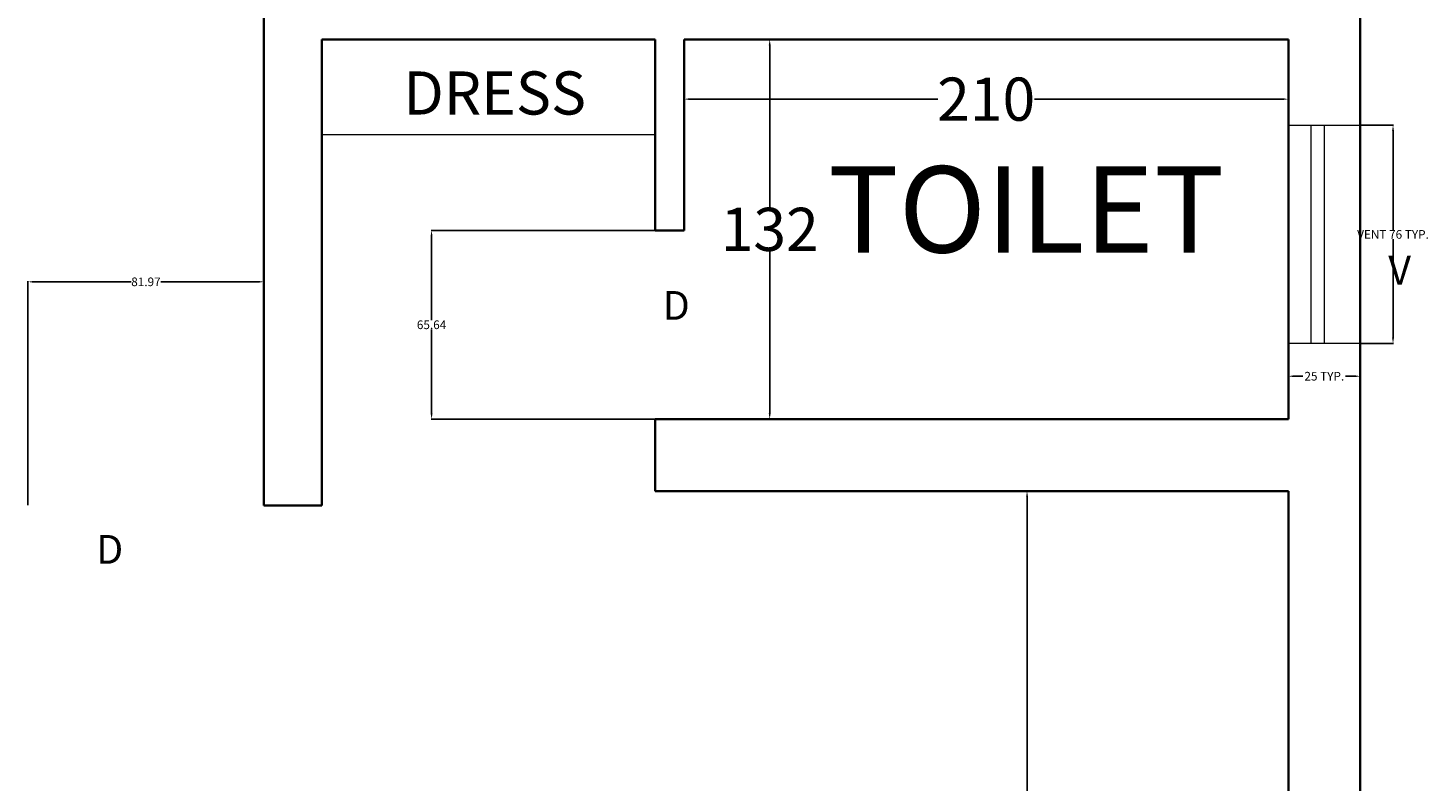
# Model space of a CAD drawing. Units: centimetres. Extents: x -121 to 3851, y -16 to 1180.
# Tile 15 of 16: x 3304 to 3791, y 320 to 582. Entities that reach past the tile are written whole.
import ezdxf

# ---------------------------------------------------------------- set-up
doc = ezdxf.new("R2010")
doc.units = ezdxf.units.CM
doc.header["$MEASUREMENT"] = 0
for name, color, linetype, lineweight in [('A-ANNO-DIMS', 2, 'Continuous', 18), ('A-ANNO-IDEN', 3, 'Continuous', 13), ('A-AREA-IDEN', 3, 'Continuous', 18), ('A-FLOR-CASE', 9, 'Continuous', 18), ('A-GLAZ', 4, 'Continuous', 18), ('A-WALL', 7, 'Continuous', 35)]:
    doc.layers.add(name, color=color, linetype=linetype, lineweight=lineweight)
doc.styles.get("Standard").update_dxf_attribs({"font": 'arial.ttf'})
doc.dimstyles.get("Standard").update_dxf_attribs({"dimtxt": 3, "dimasz": 2, "dimexe": 0.18, "dimexo": 0.0625, "dimgap": 0.09, "dimtad": 0, "dimtih": 1, "dimtoh": 1, "dimdec": 0, "dimzin": 0, "dimdsep": 46, "dimtxsty": 'Standard', "dimcen": 0.09, "dimadec": 0, "dimazin": 0, "dimtfac": 1, "dimtdec": 0, "dimtofl": 0, "dimtmove": 0, "dimatfit": 3, "dimfxl": 1, "dimtolj": 1, "dimtzin": 0, "dimarcsym": 0})

# ---------------------------------------------------------------- blocks, each defined once
blk = doc.blocks.new('*D14')
at = {"layer": 'A-ANNO-DIMS', "color": 0, "lineweight": -2, "transparency": 16777216}
for p, q in [((3562.02, 575.72), (3562.02, 519.48)), ((3562.09, 577.72), (3562.2, 577.72)), ((3562.02, 447.72), (3562.02, 503.97)), ((3562.09, 445.72), (3562.2, 445.72))]:
    blk.add_line(p, q, dxfattribs=at)
at = {"layer": 'A-ANNO-DIMS', "color": 0, "transparency": 16777216}
for points in [[(3561.69, 575.72), (3562.36, 575.72), (3562.02, 577.72)], [(3561.69, 447.72), (3562.36, 447.72), (3562.02, 445.72)]]:
    blk.add_solid(points, dxfattribs=at)
at = {"layer": 'Defpoints', "color": 0, "transparency": 16777216}
for p in [(3562.02, 577.72), (3562.02, 445.72), (3562.02, 445.72)]:
    blk.add_point(p, dxfattribs=at)
at = {"layer": 'A-ANNO-DIMS', "color": 0, "transparency": 16777216, "insert": (3562.02, 511.72), "char_height": 3, "attachment_point": 5}
blk.add_mtext('\\A1;{\\H5x;132}', dxfattribs=at)
blk = doc.blocks.new('*D15')
at = {"layer": 'A-ANNO-DIMS', "color": 0, "lineweight": -2, "transparency": 16777216}
for p, q in [((3532.26, 552.16), (3532.26, 557.17)), ((3534.26, 556.99), (3620.5, 556.99)), ((3740.26, 556.99), (3654.03, 556.99)), ((3742.26, 552.16), (3742.26, 557.17))]:
    blk.add_line(p, q, dxfattribs=at)
at = {"layer": 'A-ANNO-DIMS', "color": 0, "transparency": 16777216}
for points in [[(3534.26, 557.33), (3534.26, 556.66), (3532.26, 556.99)], [(3740.26, 557.33), (3740.26, 556.66), (3742.26, 556.99)]]:
    blk.add_solid(points, dxfattribs=at)
at = {"layer": 'Defpoints', "color": 0, "transparency": 16777216}
for p in [(3742.26, 556.99), (3532.26, 552.1), (3742.26, 552.1)]:
    blk.add_point(p, dxfattribs=at)
at = {"layer": 'A-ANNO-DIMS', "color": 0, "transparency": 16777216, "insert": (3637.26, 556.99), "char_height": 3, "attachment_point": 5}
blk.add_mtext('\\A1;{\\H5x;210}', dxfattribs=at)
blk = doc.blocks.new('*D17')
at = {"layer": 'A-ANNO-DIMS', "color": 0, "lineweight": -2, "transparency": 16777216}
for p, q in [((3651.46, 418.72), (3651.46, 281.03)), ((3651.53, 420.72), (3651.64, 420.72)), ((3651.46, 122.72), (3651.46, 260.41)), ((3651.53, 120.72), (3651.64, 120.72))]:
    blk.add_line(p, q, dxfattribs=at)
at = {"layer": 'A-ANNO-DIMS', "color": 0, "transparency": 16777216}
for points in [[(3651.13, 418.72), (3651.8, 418.72), (3651.46, 420.72)], [(3651.13, 122.72), (3651.8, 122.72), (3651.46, 120.72)]]:
    blk.add_solid(points, dxfattribs=at)
at = {"layer": 'Defpoints', "color": 0, "transparency": 16777216}
for p in [(3651.46, 420.72), (3651.46, 120.72), (3651.46, 120.72)]:
    blk.add_point(p, dxfattribs=at)
at = {"layer": 'A-ANNO-DIMS', "color": 0, "transparency": 16777216, "insert": (3651.46, 270.72), "char_height": 3, "attachment_point": 5}
blk.add_mtext('\\A1;{\\H6.66667x;300}', dxfattribs=at)
blk = doc.blocks.new('VENT-76CM')
for p, q in [((7.77, 75.86), (7.77, 0)), ((12.5, 75.86), (12.5, 0))]:
    blk.add_line(p, q)
blk.add_lwpolyline([(0, 75.86), (25, 75.86), (25, 0), (0, 0)], close=True)
blk = doc.blocks.new('*D31')
at = {"layer": 'A-ANNO-DIMS', "color": 0, "lineweight": -2, "transparency": 16777216}
for p, q in [((3767.33, 547.9), (3778.82, 547.9)), ((3778.64, 545.9), (3778.64, 511.59)), ((3778.64, 474.03), (3778.64, 508.34)), ((3767.33, 472.03), (3778.82, 472.03))]:
    blk.add_line(p, q, dxfattribs=at)
at = {"layer": 'A-ANNO-DIMS', "color": 0, "transparency": 16777216}
for points in [[(3778.31, 545.9), (3778.98, 545.9), (3778.64, 547.9)], [(3778.31, 474.03), (3778.98, 474.03), (3778.64, 472.03)]]:
    blk.add_solid(points, dxfattribs=at)
at = {"layer": 'Defpoints', "color": 0, "transparency": 16777216}
for p in [(3767.26, 547.9), (3778.64, 547.9), (3767.26, 472.03)]:
    blk.add_point(p, dxfattribs=at)
at = {"layer": 'A-ANNO-DIMS', "color": 0, "transparency": 16777216, "insert": (3778.64, 509.96), "char_height": 3, "attachment_point": 5}
blk.add_mtext('\\A1;VENT 76 TYP.', dxfattribs=at)
blk = doc.blocks.new('*D32')
at = {"layer": 'A-ANNO-DIMS', "color": 0, "lineweight": -2, "transparency": 16777216}
for p, q in [((3742.26, 471.97), (3742.26, 460.47)), ((3767.26, 471.97), (3767.26, 460.47)), ((3744.26, 460.65), (3747.35, 460.65)), ((3765.26, 460.65), (3762.18, 460.65))]:
    blk.add_line(p, q, dxfattribs=at)
at = {"layer": 'A-ANNO-DIMS', "color": 0, "transparency": 16777216}
for points in [[(3744.26, 460.99), (3744.26, 460.32), (3742.26, 460.65)], [(3765.26, 460.99), (3765.26, 460.32), (3767.26, 460.65)]]:
    blk.add_solid(points, dxfattribs=at)
at = {"layer": 'Defpoints', "color": 0, "transparency": 16777216}
for p in [(3742.26, 472.03), (3767.26, 472.03), (3767.26, 460.65)]:
    blk.add_point(p, dxfattribs=at)
at = {"layer": 'A-ANNO-DIMS', "color": 0, "transparency": 16777216, "insert": (3754.76, 460.65), "char_height": 3, "attachment_point": 5}
blk.add_mtext('\\A1;25 TYP.', dxfattribs=at)
blk = doc.blocks.new('*D72')
at = {"layer": 'A-ANNO-DIMS', "color": 0, "lineweight": -2, "transparency": 16777216}
for p, q in [((3304.26, 415.79), (3304.26, 493.65)), ((3306.26, 493.47), (3340.1, 493.47)), ((3384.23, 493.47), (3350.4, 493.47)), ((3386.23, 415.79), (3386.23, 493.65))]:
    blk.add_line(p, q, dxfattribs=at)
at = {"layer": 'A-ANNO-DIMS', "color": 0, "transparency": 16777216}
for points in [[(3306.26, 493.81), (3306.26, 493.14), (3304.26, 493.47)], [(3384.23, 493.81), (3384.23, 493.14), (3386.23, 493.47)]]:
    blk.add_solid(points, dxfattribs=at)
at = {"layer": 'Defpoints', "color": 0, "transparency": 16777216}
for p in [(3386.23, 493.47), (3304.26, 415.72), (3386.23, 415.72)]:
    blk.add_point(p, dxfattribs=at)
at = {"layer": 'A-ANNO-DIMS', "color": 0, "transparency": 16777216, "insert": (3345.25, 493.47), "char_height": 3, "attachment_point": 5}
blk.add_mtext('\\A1;81.97', dxfattribs=at)
blk = doc.blocks.new('*D80')
at = {"layer": 'A-ANNO-DIMS', "color": 0, "lineweight": -2, "transparency": 16777216}
for p, q in [((3522.2, 511.36), (3444.33, 511.36)), ((3444.51, 509.36), (3444.51, 480.17)), ((3444.51, 447.72), (3444.51, 476.92)), ((3522.2, 445.72), (3444.33, 445.72))]:
    blk.add_line(p, q, dxfattribs=at)
at = {"layer": 'A-ANNO-DIMS', "color": 0, "transparency": 16777216}
for points in [[(3444.18, 509.36), (3444.85, 509.36), (3444.51, 511.36)], [(3444.18, 447.72), (3444.85, 447.72), (3444.51, 445.72)]]:
    blk.add_solid(points, dxfattribs=at)
at = {"layer": 'Defpoints', "color": 0, "transparency": 16777216}
for p in [(3444.51, 511.36), (3522.26, 511.36), (3522.26, 445.72)]:
    blk.add_point(p, dxfattribs=at)
at = {"layer": 'A-ANNO-DIMS', "color": 0, "transparency": 16777216, "insert": (3444.51, 478.54), "char_height": 3, "attachment_point": 5}
blk.add_mtext('\\A1;65.64', dxfattribs=at)

msp = doc.modelspace()

# ---------------------------------------------------------------- linework, layer by layer
at = {"layer": 'A-FLOR-CASE'}
msp.add_line((3522.2642, 544.5435), (3406.327, 544.5435), dxfattribs=at)
at = {"layer": 'A-WALL'}
for p, q in [((3767.2642, 911.7228), (3767.2642, 95.7228)), ((3406.327, 577.7228), (3522.2642, 577.7228)), ((3522.2642, 577.7228), (3522.2642, 511.3642)), ((3532.2642, 577.7228), (3742.2642, 577.7228)), ((3532.2642, 577.7228), (3532.2642, 511.3642)), ((3742.2642, 577.7228), (3742.2642, 445.7228)), ((3532.2642, 511.3642), (3522.2642, 511.3642)), ((3522.2642, 445.7228), (3742.2642, 445.7228)), ((3522.2642, 445.7228), (3522.2642, 420.7228)), ((3522.2642, 420.7228), (3742.2642, 420.7228)), ((3742.2642, 420.7228), (3742.2642, 120.7228)), ((3386.2335, 415.7228), (3406.327, 415.7228))]:
    msp.add_line(p, q, dxfattribs=at)
for points in [[(3406.327, 592.7228), (3386.2335, 592.7228), (3386.2335, 415.7228)], [(3406.327, 415.7228), (3406.327, 577.7228)]]:
    msp.add_lwpolyline(points, dxfattribs=at)

# ---------------------------------------------------------------- block references
at = {"layer": 'A-GLAZ'}
msp.add_blockref('VENT-76CM', (3742.264, 472.0317), dxfattribs=at)

# ---------------------------------------------------------------- texts
at = {"layer": 'A-ANNO-IDEN', "char_height": 10, "attachment_point": 1}
for s, insert in [('V', (3777.014, 502.5183)), ('D', (3524.8639, 490.2699)), ('D', (3327.9743, 405.4487))]:
    msp.add_mtext_dynamic_manual_height_columns(s, width=55.718495, gutter_width=1, heights=[0], dxfattribs=dict(at, insert=insert))
at = {"layer": 'A-AREA-IDEN', "attachment_point": 1}
for s, width, insert, char_height in [('DRESS', 14.894434, (3434.6907, 566.6266), 15), ('TOILET', 114.065148, (3582.3236, 533.6636), 30)]:
    msp.add_mtext_dynamic_manual_height_columns(s, width=width, gutter_width=1, heights=[0], dxfattribs=dict(at, insert=insert, char_height=char_height))

# ---------------------------------------------------------------- dimensions: what is measured, and where the dimension line sits
at = {"layer": 'A-ANNO-DIMS'}
for base, p1, p2, text, override, picture, middle in [((3562.0228, 445.7228), (3562.0228, 577.7228), (3562.0228, 445.7228), '{\\H5x;<>}', {"dimclrd": 0, "dimclre": 0, "dimclrt": 0}, '*D14', (3562.0228, 511.7228)), ((3778.6438, 547.8954), (3767.2642, 472.0314), (3767.2642, 547.8954), 'VENT <> TYP.', {"dimdec": 0, "dimlfac": 1, "dimrnd": 0, "dimzin": 0, "dimdsep": 46, "dimlunit": 2}, '*D31', (3778.6438, 509.9634)), ((3651.464, 120.7228), (3651.464, 420.7228), (3651.464, 120.7228), '{\\H6.66667x;<>}', {"dimclrd": 0, "dimclre": 0, "dimclrt": 0}, '*D17', (3651.464, 270.7228))]:
    dim = msp.add_linear_dim(base=base, p1=p1, p2=p2, angle=90, text=text, dimstyle='Standard', override=override, dxfattribs=at)
    dim.commit()
    dim.dimension.update_dxf_attribs({"geometry": picture, "text_midpoint": middle})
for base, p1, p2, text, override, picture, middle in [((3742.2642, 556.9932), (3532.2642, 552.099), (3742.2642, 552.099), '{\\H5x;<>}', {"dimclrd": 0, "dimclre": 0, "dimclrt": 0}, '*D15', (3637.2642, 556.9932)), ((3767.2642, 460.6518), (3742.2642, 472.0314), (3767.2642, 472.0314), '<> TYP.', {"dimdec": 0, "dimlfac": 1, "dimrnd": 0, "dimzin": 0, "dimdsep": 46, "dimlunit": 2}, '*D32', (3754.7642, 460.6518))]:
    dim = msp.add_linear_dim(base=base, p1=p1, p2=p2, text=text, dimstyle='Standard', override=override, dxfattribs=at)
    dim.commit()
    dim.dimension.update_dxf_attribs({"geometry": picture, "text_midpoint": middle})
for base, p1, p2, angle, picture, middle in [((3444.5142, 511.3642), (3522.2642, 445.7228), (3522.2642, 511.3642), 90, '*D80', (3444.5142, 478.5435)), ((3386.2335, 493.4728), (3304.2642, 415.7228), (3386.2335, 415.7228), 0, '*D72', (3345.2488, 493.4728))]:
    dim = msp.add_linear_dim(base=base, p1=p1, p2=p2, angle=angle, dimstyle='Standard', override={"dimdec": 2, "dimlfac": 1, "dimrnd": 0, "dimzin": 0, "dimdsep": 46, "dimlunit": 2}, dxfattribs=at)
    dim.commit()
    dim.dimension.update_dxf_attribs({"geometry": picture, "text_midpoint": middle})

doc.saveas('drawing.dxf')
